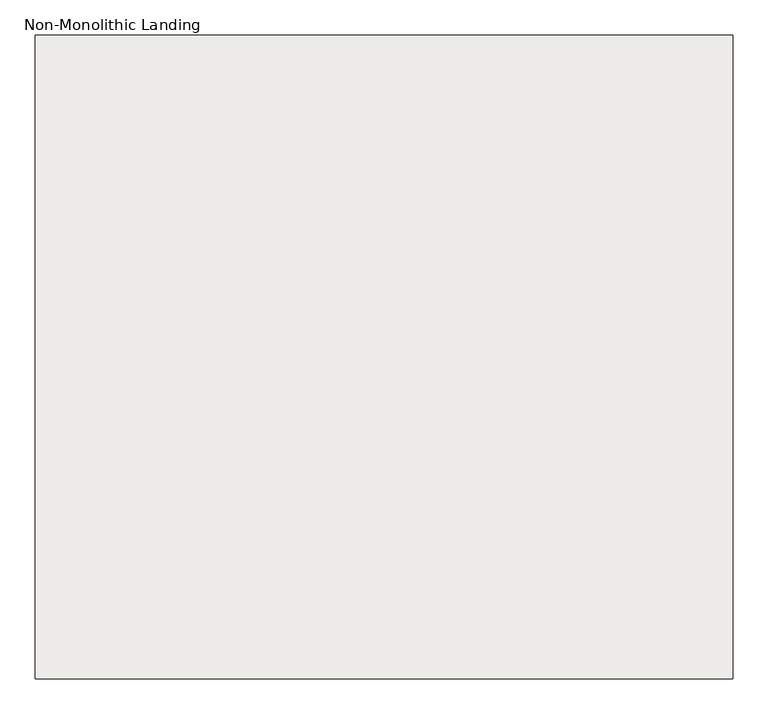
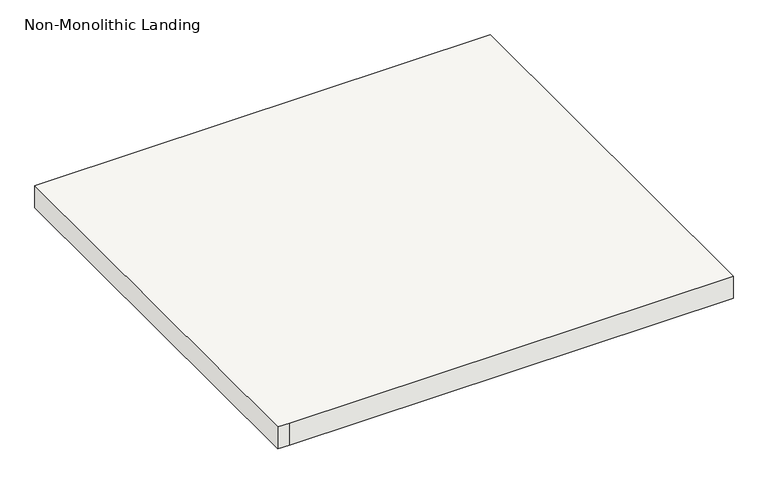
"""IFC4 building model written with IfcOpenShell, lengths in millimetres: slab geometry, Non-Monolithic Landing."""

from ifc_helpers import new_model, si_unit, origin, place, context, project, spatial, faceted_brep, source, transform, mapped, element, save


def non_monolithic_landing_440175ab(model_context):
    return source(origin(), model_context, "Body", "Brep", [
        faceted_brep([(3609.7430349, 2997.8555142, 5060.95), (3609.7430349, 2972.4555142, 5035.55), (2695.3430349, 2972.4555142, 5035.55), (2695.3430349, 2997.8555142, 5060.95), (2644.5430349, 2997.8555142, 5080.0), (2619.1430349, 2997.8555142, 5080.0), (2619.1430349, 2083.4555142, 5080.0), (2644.5430349, 2083.4555142, 5080.0), (3609.7430349, 2083.4555142, 5080.0), (3609.7430349, 2997.8555142, 5080.0), (2695.3430349, 2972.4555142, 5029.2), (3609.7430349, 2972.4555142, 5029.2), (3609.7430349, 2083.4555142, 5029.2), (2644.5430349, 2083.4555142, 5029.2), (2619.1430349, 2083.4555142, 5029.2), (2619.1430349, 2997.8555142, 5029.2), (2644.5430349, 2997.8555142, 5029.2), (2695.3430349, 2997.8555142, 5029.2)], [[[0, 1, 2, 3]], [[4, 5, 6, 7, 8, 9]], [[10, 11, 12, 13, 14, 15, 16, 17]], [[11, 10, 2, 1]], [[10, 17, 3, 2]], [[4, 9, 0, 3, 17, 16]], [[5, 4, 16, 15]], [[6, 5, 15, 14]], [[7, 6, 14, 13]], [[8, 7, 13, 12]], [[9, 8, 12, 11, 1, 0]]]),
    ])


if __name__ == "__main__":
    model = new_model("IFC4")
    model_context = context("Model", 3, world=origin())
    ifc_project = project(units=[si_unit("LENGTHUNIT", "METRE", prefix="MILLI")], contexts=[model_context])
    site = spatial("IfcSite", under=ifc_project)
    building = spatial("IfcBuilding", under=site)
    placement = place(None, origin())
    non_monolithic_landing_shape = non_monolithic_landing_440175ab(model_context)
    element("IfcSlab", 1, ObjectType="Non-Monolithic Landing", at=placement, inside=building, context=model_context, shape_type="MappedRepresentation", body=[
        mapped(non_monolithic_landing_shape, transform((0.0, 0.0, 0.0), x_axis=(1.0, 0.0, 0.0), y_axis=(0.0, 1.0, 0.0), z_axis=(0.0, 0.0, 1.0))),
    ])
    save(model, "model.ifc")
